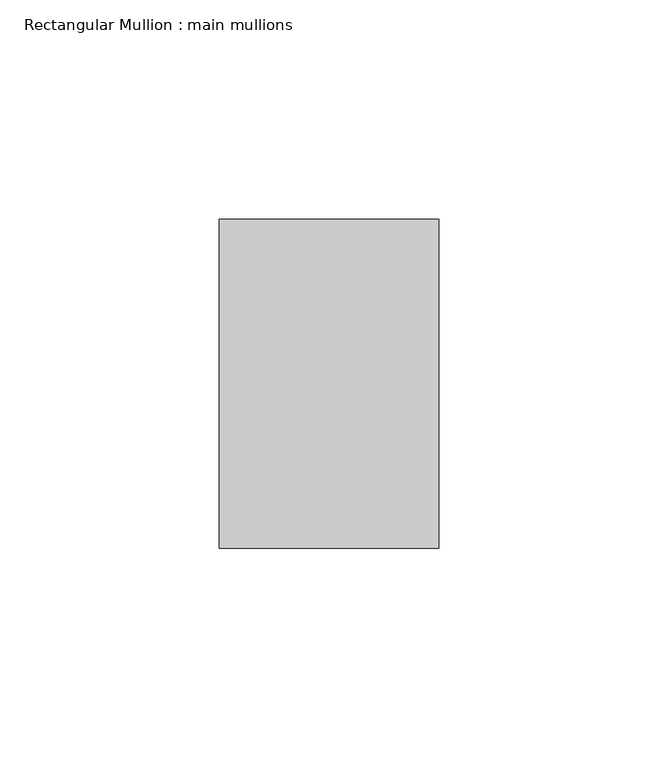
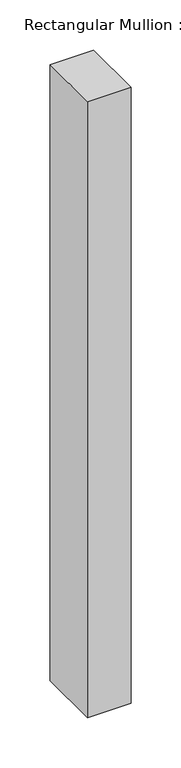
"""IFC4 building model written with IfcOpenShell, lengths in millimetres: member geometry, Rectangular Mullion : main mullions."""

from ifc_helpers import new_model, si_unit, frame, origin, place, context, project, spatial, polyline, outline, extrude, source, transform, mapped, element, save


def rectangular_mullion_main_mullions_bcbd968b(model_context):
    return source(origin(), model_context, "Body", "SweptSolid", [
        extrude(outline(polyline([(25.0, 37.5), (25.0, -37.5), (-25.0, -37.5), (-25.0, 37.5), (25.0, 37.5)])), frame((0.0, 0.0, -750.0), z_axis=(0.0, 0.0, 1.0), x_axis=(1.0, 0.0, 0.0)), (0.0, 0.0, 1.0), 750.0),
    ])


if __name__ == "__main__":
    model = new_model("IFC4")
    model_context = context("Model", 3, world=origin())
    ifc_project = project(units=[si_unit("LENGTHUNIT", "METRE", prefix="MILLI")], contexts=[model_context])
    site = spatial("IfcSite", under=ifc_project)
    building = spatial("IfcBuilding", under=site)
    placement = place(None, origin())
    rectangular_mullion_main_mullions_shape = rectangular_mullion_main_mullions_bcbd968b(model_context)
    element("IfcMember", 1, ObjectType="Rectangular Mullion : main mullions", at=placement, inside=building, context=model_context, shape_type="MappedRepresentation", body=[
        mapped(rectangular_mullion_main_mullions_shape, transform((0.0, 0.0, 0.0), x_axis=(1.0, 0.0, 0.0), y_axis=(0.0, 1.0, 0.0), z_axis=(0.0, 0.0, 1.0))),
    ])
    save(model, "model.ifc")

# Revit data of these elements
# Type "Rectangular Mullion : main mullions"
#   built-in parameter 1007304 = 0.246063 (stored number, unit not read)
#   built-in parameter 1007301 = 0.082021 (stored number, unit not read)
#   built-in parameter 1007300 = 0.082021 (stored number, unit not read)
# Element 1 (IfcMember, "Rectangular Mullion : main mullions")
#   Materials on its faces: "Aluminum"
# Materials
#   "Aluminum": class "Metal", colour RGB 136 136 136, transparency 0, Description = "Aluminum 6061", Cost = 0
